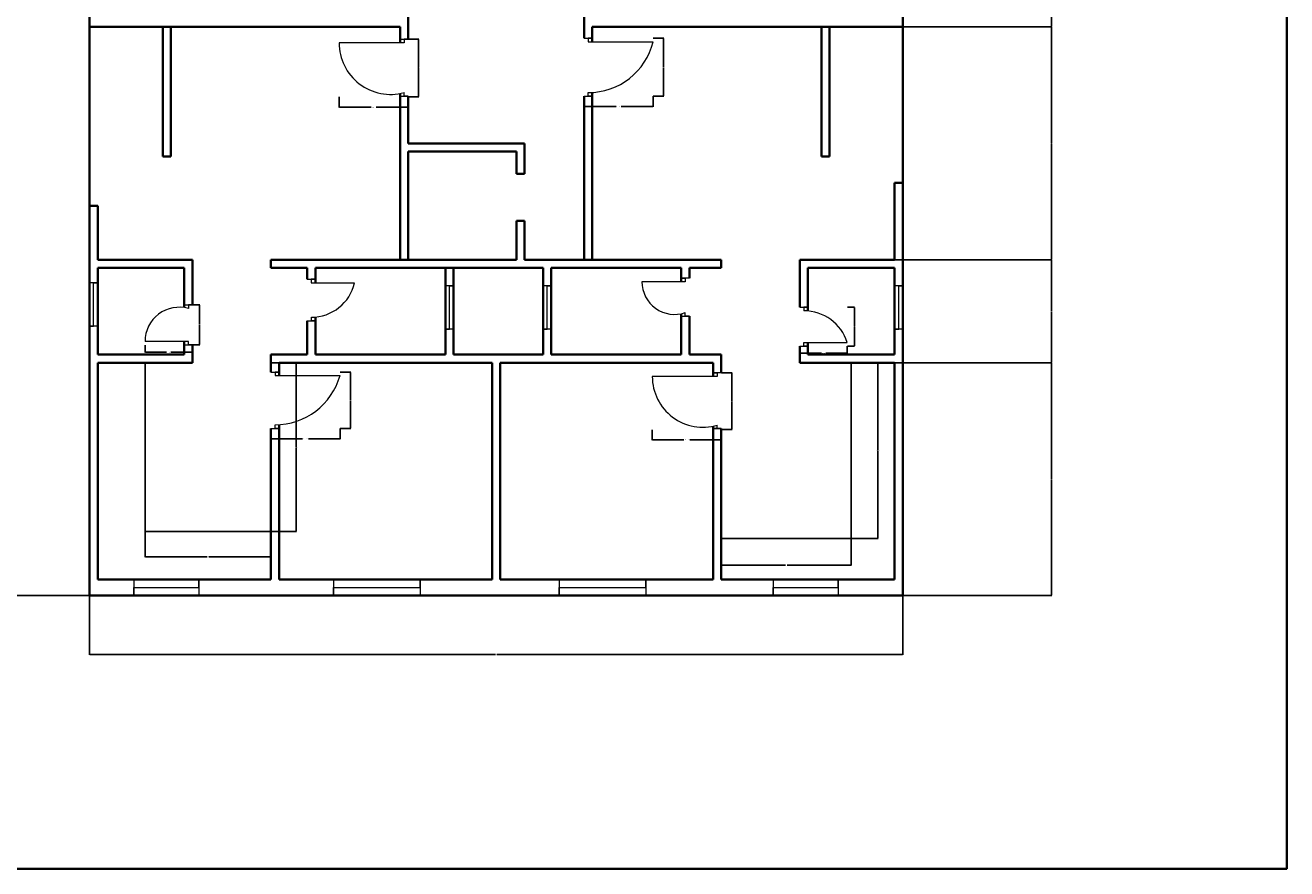
# Model space of a CAD drawing. Units: inches. Extents: x 2043 to 3387, y 1535 to 2797.
# Tile 4 of 7: x 2688 to 3387, y 1535 to 2002. Entities that reach past the tile are written whole.
import ezdxf

# ---------------------------------------------------------------- set-up
doc = ezdxf.new("R2010")
doc.units = ezdxf.units.IN
for name, color, linetype, lineweight in [('A-ANNO-DIMS', 2, 'Continuous', 18), ('A-ANNO-TTLB', 7, 'Continuous', 35), ('A-DOOR', 3, 'Continuous', 18), ('A-FLOR-FIXT', 9, 'Continuous', 25), ('A-GLAZ', 4, 'Continuous', 18), ('A-WALL', 7, 'Continuous', 35)]:
    doc.layers.add(name, color=color, linetype=linetype, lineweight=lineweight)
doc.styles.get("Standard").update_dxf_attribs({"font": 'arial.ttf'})
doc.dimstyles.get("Standard").update_dxf_attribs({"dimtxt": 0.18, "dimasz": 0.18, "dimexe": 0.18, "dimexo": 0.0625, "dimgap": 0.09, "dimtad": 0, "dimtih": 1, "dimtoh": 1, "dimdec": 4, "dimzin": 0, "dimdsep": 46, "dimtxsty": 'Standard', "dimcen": 0.09, "dimadec": 0, "dimazin": 0, "dimtfac": 1, "dimtdec": 4, "dimtofl": 0, "dimtmove": 0, "dimatfit": 3, "dimfxl": 1, "dimtolj": 1, "dimtzin": 0, "dimarcsym": 0})

# ---------------------------------------------------------------- blocks, each defined once
blk = doc.blocks.new('DOOR-36-ENTRY-SW')
for p, q in [((36, 29.57), (0, 29.57)), ((33.75, 31.57), (38.25, 31.57)), ((38.25, 31.57), (36, 31.57)), ((36, 31.57), (36, 29.57)), ((36, 0), (36, 2)), ((33.75, 0), (38.25, 0)), ((38.25, 0), (36, 0))]:
    blk.add_line(p, q)
blk.add_arc((28.56, 29.57), 28.56, 180, 285.10352)
blk = doc.blocks.new('DOOR-36-ENTRY-SE')
for p, q in [((0, 32.19), (4.5, 32.19)), ((4.5, 32.19), (2.25, 32.19)), ((2.25, 32.19), (2.25, 30.19)), ((2.25, 30.19), (38.25, 30.19)), ((2.25, 0), (2.25, 2)), ((0, 0), (4.5, 0)), ((4.5, 0), (2.25, 0))]:
    blk.add_line(p, q)
blk.add_arc((2.25, 39.08), 37.08, 270, 346.11724)
blk = doc.blocks.new('DOOR-24-WC-SW')
for p, q in [((21.75, 22.19), (26.25, 22.19)), ((26.25, 22.19), (24, 22.19)), ((24, 22.19), (24, 20.19)), ((24, 2), (0, 2)), ((21.75, 0), (26.25, 0)), ((24, 0), (24, 2)), ((26.25, 0), (24, 0))]:
    blk.add_line(p, q)
blk.add_arc((18.89, 2), 18.89, 74.30449, 180)
blk = doc.blocks.new('DOOR-24-BATH-SW')
for p, q in [((0, 23.05), (4.63, 23.05)), ((4.63, 23.05), (2.31, 23.05)), ((2.31, 23.05), (2.31, 21.05)), ((2.31, 21.05), (26.31, 21.05)), ((2.34, 0), (2.34, 2)), ((0.06, 0), (4.63, 0)), ((4.63, 0), (2.34, 0))]:
    blk.add_line(p, q)
blk.add_arc((2.34, 26.6), 24.6, 270, 346.95638)
blk = doc.blocks.new('DOOR-24-BATH-SE')
for p, q in [((26.25, 21.13), (21.75, 21.13)), ((21.75, 21.13), (24, 21.13)), ((24, 21.13), (24, 19.13)), ((24, 19.13), (0, 19.13)), ((24, 0), (24, 2)), ((21.75, 0), (26.25, 0)), ((26.25, 0), (24, 0))]:
    blk.add_line(p, q)
blk.add_arc((18.12, 19.13), 18.12, 180, 288.95077)
blk = doc.blocks.new('DOOR-24-WC-SE')
for p, q in [((0, 21.53), (4.5, 21.53)), ((4.5, 21.53), (2.25, 21.53)), ((2.25, 21.53), (2.25, 19.53)), ((0, 0), (4.5, 0)), ((2.25, 0), (2.25, 2)), ((2.25, 2), (26.25, 2)), ((4.5, 0), (2.25, 0))]:
    blk.add_line(p, q)
blk.add_arc((2.25, -5.66), 25.19, 17.71019, 90)
blk = doc.blocks.new('DOOR-36-BED-SE')
for p, q in [((36, 28.83), (0, 28.83)), ((38.25, 30.83), (33.75, 30.83)), ((33.75, 30.83), (36, 30.83)), ((36, 30.83), (36, 28.83)), ((33.75, 0), (38.25, 0)), ((38.25, 0), (33.75, 0)), ((33.75, 0), (36, 0)), ((36, 0), (36, 2))]:
    blk.add_line(p, q)
blk.add_arc((28, 28.83), 28, 180, 286.60822)
blk = doc.blocks.new('DOOR-36-BED-SW')
for p, q in [((0, 31.2), (4.5, 31.2)), ((4.5, 31.2), (2.25, 31.2)), ((2.25, 31.2), (2.25, 29.2)), ((2.25, 29.2), (38.25, 29.2)), ((0, 0), (4.5, 0)), ((2.25, 0), (2.25, 2)), ((4.5, 0), (2.25, 0))]:
    blk.add_line(p, q)
blk.add_arc((2.25, 39.42), 37.42, 270, 344.14237)
blk = doc.blocks.new('COUNTER-L-SW')
for p, q in [((0, 93.54), (0, 0)), ((0, 0), (69.75, 0))]:
    blk.add_line(p, q)
blk = doc.blocks.new('COUNTER-L-SE')
for p, q in [((72, 97.45), (72, 0)), ((72, 0), (0, 0))]:
    blk.add_line(p, q)
blk = doc.blocks.new('WIN-48-PLAN')
for p, q in [((0, 9), (0, 0)), ((48, 4.5), (48, 9)), ((48, 9), (48, 0)), ((0, 0), (0, 4.5)), ((0, 4.5), (48, 4.5))]:
    blk.add_line(p, q)
blk = doc.blocks.new('VENT-24-PLAN')
for p, q in [((0, 24), (4.5, 24)), ((4.5, 24), (2.25, 24)), ((2.25, 24), (2.25, 0)), ((2.25, 0), (0, 0)), ((0, 0), (4.5, 0))]:
    blk.add_line(p, q)
blk = doc.blocks.new('WIN-36-PLAN')
for p, q in [((0, 9), (0, 0)), ((36, 4.5), (36, 9)), ((36, 9), (36, 0)), ((0, 0), (0, 4.5)), ((0, 4.5), (36, 4.5))]:
    blk.add_line(p, q)
blk = doc.blocks.new('*D53')
at = {"layer": 'A-ANNO-DIMS', "color": 0, "lineweight": -2, "transparency": 16777216}
for p, q in [((2754.46, 1824.65), (2754.46, 1820.59)), ((2780.71, 1824.65), (2780.71, 1820.59)), ((2754.64, 1820.77), (2766.4, 1820.77)), ((2780.53, 1820.77), (2768.77, 1820.77))]:
    blk.add_line(p, q, dxfattribs=at)
at = {"layer": 'A-ANNO-DIMS', "color": 0, "transparency": 16777216}
for points in [[(2754.64, 1820.8), (2754.64, 1820.74), (2754.46, 1820.77)], [(2780.53, 1820.8), (2780.53, 1820.74), (2780.71, 1820.77)]]:
    blk.add_solid(points, dxfattribs=at)
at = {"layer": 'Defpoints', "color": 0, "transparency": 16777216}
for p in [(2754.46, 1824.71), (2780.71, 1824.71), (2780.71, 1820.77)]:
    blk.add_point(p, dxfattribs=at)
at = {"layer": 'A-ANNO-DIMS', "color": 0, "transparency": 16777216, "insert": (2767.58, 1820.77), "char_height": 0.18, "attachment_point": 5}
blk.add_mtext('\\A1;WC DOOR 26 TYP.', dxfattribs=at)
blk = doc.blocks.new('*D54')
at = {"layer": 'A-ANNO-DIMS', "color": 0, "lineweight": -2, "transparency": 16777216}
for p, q in [((2780.77, 1846.9), (2784.83, 1846.9)), ((2784.65, 1846.72), (2784.65, 1835.98)), ((2784.65, 1824.89), (2784.65, 1835.62)), ((2780.77, 1824.71), (2784.83, 1824.71))]:
    blk.add_line(p, q, dxfattribs=at)
at = {"layer": 'A-ANNO-DIMS', "color": 0, "transparency": 16777216}
for points in [[(2784.62, 1846.72), (2784.68, 1846.72), (2784.65, 1846.9)], [(2784.62, 1824.89), (2784.68, 1824.89), (2784.65, 1824.71)]]:
    blk.add_solid(points, dxfattribs=at)
at = {"layer": 'Defpoints', "color": 0, "transparency": 16777216}
for p in [(2780.71, 1846.9), (2784.65, 1846.9), (2780.71, 1824.71)]:
    blk.add_point(p, dxfattribs=at)
at = {"layer": 'A-ANNO-DIMS', "color": 0, "transparency": 16777216, "insert": (2784.65, 1835.8), "char_height": 0.18, "attachment_point": 5}
blk.add_mtext('\\A1;22 TYP.', dxfattribs=at)
blk = doc.blocks.new('*D55')
at = {"layer": 'A-ANNO-DIMS', "color": 0, "lineweight": -2, "transparency": 16777216}
for p, q in [((3117.21, 1824.03), (3117.21, 1819.98)), ((3117.39, 1820.16), (3129.15, 1820.16)), ((3143.28, 1820.16), (3131.52, 1820.16)), ((3143.46, 1824.03), (3143.46, 1819.98))]:
    blk.add_line(p, q, dxfattribs=at)
at = {"layer": 'A-ANNO-DIMS', "color": 0, "transparency": 16777216}
for points in [[(3117.39, 1820.19), (3117.39, 1820.13), (3117.21, 1820.16)], [(3143.28, 1820.19), (3143.28, 1820.13), (3143.46, 1820.16)]]:
    blk.add_solid(points, dxfattribs=at)
at = {"layer": 'Defpoints', "color": 0, "transparency": 16777216}
for p in [(3117.21, 1824.1), (3143.46, 1824.1), (3143.46, 1820.16)]:
    blk.add_point(p, dxfattribs=at)
at = {"layer": 'A-ANNO-DIMS', "color": 0, "transparency": 16777216, "insert": (3130.33, 1820.16), "char_height": 0.18, "attachment_point": 5}
blk.add_mtext('\\A1;WC DOOR 26 TYP.', dxfattribs=at)
blk = doc.blocks.new('*D56')
at = {"layer": 'A-ANNO-DIMS', "color": 0, "lineweight": -2, "transparency": 16777216}
for p, q in [((3143.52, 1845.63), (3147.58, 1845.63)), ((3147.4, 1845.45), (3147.4, 1835.04)), ((3147.4, 1824.28), (3147.4, 1834.68)), ((3143.52, 1824.1), (3147.58, 1824.1))]:
    blk.add_line(p, q, dxfattribs=at)
at = {"layer": 'A-ANNO-DIMS', "color": 0, "transparency": 16777216}
for points in [[(3147.37, 1845.45), (3147.43, 1845.45), (3147.4, 1845.63)], [(3147.37, 1824.28), (3147.43, 1824.28), (3147.4, 1824.1)]]:
    blk.add_solid(points, dxfattribs=at)
at = {"layer": 'Defpoints', "color": 0, "transparency": 16777216}
for p in [(3143.46, 1845.63), (3147.4, 1845.63), (3143.46, 1824.1)]:
    blk.add_point(p, dxfattribs=at)
at = {"layer": 'A-ANNO-DIMS', "color": 0, "transparency": 16777216, "insert": (3147.4, 1834.86), "char_height": 0.18, "attachment_point": 5}
blk.add_mtext('\\A1;22 TYP.', dxfattribs=at)
blk = doc.blocks.new('*D69')
at = {"layer": 'A-ANNO-DIMS', "color": 0, "lineweight": -2, "transparency": 16777216}
for p, q in [((2861.96, 1962.12), (2861.96, 1956.27)), ((2900.21, 1962.12), (2900.21, 1956.27)), ((2862.14, 1956.45), (2879.69, 1956.45)), ((2900.03, 1956.45), (2882.48, 1956.45))]:
    blk.add_line(p, q, dxfattribs=at)
at = {"layer": 'A-ANNO-DIMS', "color": 0, "transparency": 16777216}
for points in [[(2862.14, 1956.48), (2862.14, 1956.42), (2861.96, 1956.45)], [(2900.03, 1956.48), (2900.03, 1956.42), (2900.21, 1956.45)]]:
    blk.add_solid(points, dxfattribs=at)
at = {"layer": 'Defpoints', "color": 0, "transparency": 16777216}
for p in [(2861.96, 1962.19), (2900.21, 1962.19), (2900.21, 1956.45)]:
    blk.add_point(p, dxfattribs=at)
at = {"layer": 'A-ANNO-DIMS', "color": 0, "transparency": 16777216, "insert": (2881.08, 1956.45), "char_height": 0.18, "attachment_point": 5}
blk.add_mtext('\\A1;ENTRY DOOR 38 TYP.', dxfattribs=at)
blk = doc.blocks.new('*D70')
at = {"layer": 'A-ANNO-DIMS', "color": 0, "lineweight": -2, "transparency": 16777216}
for p, q in [((2900.27, 1994.07), (2906.13, 1994.07)), ((2905.95, 1993.89), (2905.95, 1978.31)), ((2905.95, 1962.37), (2905.95, 1977.95)), ((2900.27, 1962.19), (2906.13, 1962.19))]:
    blk.add_line(p, q, dxfattribs=at)
at = {"layer": 'A-ANNO-DIMS', "color": 0, "transparency": 16777216}
for points in [[(2905.92, 1993.89), (2905.98, 1993.89), (2905.95, 1994.07)], [(2905.92, 1962.37), (2905.98, 1962.37), (2905.95, 1962.19)]]:
    blk.add_solid(points, dxfattribs=at)
at = {"layer": 'Defpoints', "color": 0, "transparency": 16777216}
for p in [(2900.21, 1994.07), (2905.95, 1994.07), (2900.21, 1962.19)]:
    blk.add_point(p, dxfattribs=at)
at = {"layer": 'A-ANNO-DIMS', "color": 0, "transparency": 16777216, "insert": (2905.95, 1978.13), "char_height": 0.18, "attachment_point": 5}
blk.add_mtext('\\A1;32 TYP.', dxfattribs=at)
blk = doc.blocks.new('*D71')
at = {"layer": 'A-ANNO-DIMS', "color": 0, "lineweight": -2, "transparency": 16777216}
for p, q in [((2997.71, 1962.44), (2997.71, 1956.58)), ((3035.96, 1962.44), (3035.96, 1956.58)), ((2997.89, 1956.76), (3015.44, 1956.76)), ((3035.78, 1956.76), (3018.23, 1956.76))]:
    blk.add_line(p, q, dxfattribs=at)
at = {"layer": 'A-ANNO-DIMS', "color": 0, "transparency": 16777216}
for points in [[(2997.89, 1956.79), (2997.89, 1956.73), (2997.71, 1956.76)], [(3035.78, 1956.79), (3035.78, 1956.73), (3035.96, 1956.76)]]:
    blk.add_solid(points, dxfattribs=at)
at = {"layer": 'Defpoints', "color": 0, "transparency": 16777216}
for p in [(2997.71, 1962.5), (3035.96, 1962.5), (3035.96, 1956.76)]:
    blk.add_point(p, dxfattribs=at)
at = {"layer": 'A-ANNO-DIMS', "color": 0, "transparency": 16777216, "insert": (3016.83, 1956.76), "char_height": 0.18, "attachment_point": 5}
blk.add_mtext('\\A1;ENTRY DOOR 38 TYP.', dxfattribs=at)
blk = doc.blocks.new('*D72')
at = {"layer": 'A-ANNO-DIMS', "color": 0, "lineweight": -2, "transparency": 16777216}
for p, q in [((3036.02, 1994.69), (3041.88, 1994.69)), ((3041.7, 1994.51), (3041.7, 1978.78)), ((3041.7, 1962.68), (3041.7, 1978.41)), ((3036.02, 1962.5), (3041.88, 1962.5))]:
    blk.add_line(p, q, dxfattribs=at)
at = {"layer": 'A-ANNO-DIMS', "color": 0, "transparency": 16777216}
for points in [[(3041.67, 1994.51), (3041.73, 1994.51), (3041.7, 1994.69)], [(3041.67, 1962.68), (3041.73, 1962.68), (3041.7, 1962.5)]]:
    blk.add_solid(points, dxfattribs=at)
at = {"layer": 'Defpoints', "color": 0, "transparency": 16777216}
for p in [(3035.96, 1994.69), (3041.7, 1994.69), (3035.96, 1962.5)]:
    blk.add_point(p, dxfattribs=at)
at = {"layer": 'A-ANNO-DIMS', "color": 0, "transparency": 16777216, "insert": (3041.7, 1978.59), "char_height": 0.18, "attachment_point": 5}
blk.add_mtext('\\A1;32 TYP.', dxfattribs=at)
blk = doc.blocks.new('*D77')
at = {"layer": 'A-ANNO-DIMS', "color": 0, "lineweight": -2, "transparency": 16777216}
for p, q in [((2824.21, 1778.46), (2824.21, 1772.61)), ((2862.46, 1778.46), (2862.46, 1772.61)), ((2824.39, 1772.79), (2841.71, 1772.79)), ((2862.28, 1772.79), (2844.95, 1772.79))]:
    blk.add_line(p, q, dxfattribs=at)
at = {"layer": 'A-ANNO-DIMS', "color": 0, "transparency": 16777216}
for points in [[(2824.39, 1772.82), (2824.39, 1772.76), (2824.21, 1772.79)], [(2862.28, 1772.82), (2862.28, 1772.76), (2862.46, 1772.79)]]:
    blk.add_solid(points, dxfattribs=at)
at = {"layer": 'Defpoints', "color": 0, "transparency": 16777216}
for p in [(2824.21, 1778.52), (2862.46, 1778.52), (2862.46, 1772.79)]:
    blk.add_point(p, dxfattribs=at)
at = {"layer": 'A-ANNO-DIMS', "color": 0, "transparency": 16777216, "insert": (2843.33, 1772.79), "char_height": 0.18, "attachment_point": 5}
blk.add_mtext('\\A1;BEDROOM DOOR 38 TYP.', dxfattribs=at)
blk = doc.blocks.new('*D78')
at = {"layer": 'A-ANNO-DIMS', "color": 0, "lineweight": -2, "transparency": 16777216}
for p, q in [((2862.52, 1809.72), (2868.38, 1809.72)), ((2868.2, 1809.54), (2868.2, 1794.3)), ((2868.2, 1778.7), (2868.2, 1793.94)), ((2862.52, 1778.52), (2868.38, 1778.52))]:
    blk.add_line(p, q, dxfattribs=at)
at = {"layer": 'A-ANNO-DIMS', "color": 0, "transparency": 16777216}
for points in [[(2868.17, 1809.54), (2868.23, 1809.54), (2868.2, 1809.72)], [(2868.17, 1778.7), (2868.23, 1778.7), (2868.2, 1778.52)]]:
    blk.add_solid(points, dxfattribs=at)
at = {"layer": 'Defpoints', "color": 0, "transparency": 16777216}
for p in [(2862.46, 1809.72), (2868.2, 1809.72), (2862.46, 1778.52)]:
    blk.add_point(p, dxfattribs=at)
at = {"layer": 'A-ANNO-DIMS', "color": 0, "transparency": 16777216, "insert": (2868.2, 1794.12), "char_height": 0.18, "attachment_point": 5}
blk.add_mtext('\\A1;31 TYP.', dxfattribs=at)
blk = doc.blocks.new('*D79')
at = {"layer": 'A-ANNO-DIMS', "color": 0, "lineweight": -2, "transparency": 16777216}
for p, q in [((3035.46, 1777.76), (3035.46, 1771.91)), ((3073.71, 1777.76), (3073.71, 1771.91)), ((3035.64, 1772.09), (3052.96, 1772.09)), ((3073.53, 1772.09), (3056.2, 1772.09))]:
    blk.add_line(p, q, dxfattribs=at)
at = {"layer": 'A-ANNO-DIMS', "color": 0, "transparency": 16777216}
for points in [[(3035.64, 1772.12), (3035.64, 1772.06), (3035.46, 1772.09)], [(3073.53, 1772.12), (3073.53, 1772.06), (3073.71, 1772.09)]]:
    blk.add_solid(points, dxfattribs=at)
at = {"layer": 'Defpoints', "color": 0, "transparency": 16777216}
for p in [(3035.46, 1777.82), (3073.71, 1777.82), (3073.71, 1772.09)]:
    blk.add_point(p, dxfattribs=at)
at = {"layer": 'A-ANNO-DIMS', "color": 0, "transparency": 16777216, "insert": (3054.58, 1772.09), "char_height": 0.18, "attachment_point": 5}
blk.add_mtext('\\A1;BEDROOM DOOR 38 TYP.', dxfattribs=at)
blk = doc.blocks.new('*D80')
at = {"layer": 'A-ANNO-DIMS', "color": 0, "lineweight": -2, "transparency": 16777216}
for p, q in [((3073.77, 1809.18), (3079.63, 1809.18)), ((3079.45, 1809), (3079.45, 1793.69)), ((3079.45, 1778), (3079.45, 1793.32)), ((3073.77, 1777.82), (3079.63, 1777.82))]:
    blk.add_line(p, q, dxfattribs=at)
at = {"layer": 'A-ANNO-DIMS', "color": 0, "transparency": 16777216}
for points in [[(3079.42, 1809), (3079.48, 1809), (3079.45, 1809.18)], [(3079.42, 1778), (3079.48, 1778), (3079.45, 1777.82)]]:
    blk.add_solid(points, dxfattribs=at)
at = {"layer": 'Defpoints', "color": 0, "transparency": 16777216}
for p in [(3073.71, 1809.18), (3079.45, 1809.18), (3073.71, 1777.82)]:
    blk.add_point(p, dxfattribs=at)
at = {"layer": 'A-ANNO-DIMS', "color": 0, "transparency": 16777216, "insert": (3079.45, 1793.5), "char_height": 0.18, "attachment_point": 5}
blk.add_mtext('\\A1;31 TYP.', dxfattribs=at)
blk = doc.blocks.new('*D85')
at = {"layer": 'A-ANNO-DIMS', "color": 0, "lineweight": -2, "transparency": 16777216}
for p, q in [((2824.27, 1814.88), (2838.42, 1814.88)), ((2838.24, 1814.7), (2838.24, 1768.29)), ((2838.24, 1721.52), (2838.24, 1767.92)), ((2824.27, 1721.34), (2838.42, 1721.34))]:
    blk.add_line(p, q, dxfattribs=at)
at = {"layer": 'A-ANNO-DIMS', "color": 0, "transparency": 16777216}
for points in [[(2838.21, 1814.7), (2838.27, 1814.7), (2838.24, 1814.88)], [(2838.21, 1721.52), (2838.27, 1721.52), (2838.24, 1721.34)]]:
    blk.add_solid(points, dxfattribs=at)
at = {"layer": 'Defpoints', "color": 0, "transparency": 16777216}
for p in [(2824.21, 1814.88), (2838.24, 1814.88), (2824.21, 1721.34)]:
    blk.add_point(p, dxfattribs=at)
at = {"layer": 'A-ANNO-DIMS', "color": 0, "transparency": 16777216, "insert": (2838.24, 1768.11), "char_height": 0.18, "attachment_point": 5}
blk.add_mtext('\\A1;COUNTER 94 TYP.', dxfattribs=at)
blk = doc.blocks.new('*D86')
at = {"layer": 'A-ANNO-DIMS', "color": 0, "lineweight": -2, "transparency": 16777216}
for p, q in [((2754.46, 1721.28), (2754.46, 1707.13)), ((2824.21, 1721.28), (2824.21, 1707.13)), ((2754.64, 1707.31), (2788.81, 1707.31)), ((2824.03, 1707.31), (2789.86, 1707.31))]:
    blk.add_line(p, q, dxfattribs=at)
at = {"layer": 'A-ANNO-DIMS', "color": 0, "transparency": 16777216}
for points in [[(2754.64, 1707.34), (2754.64, 1707.28), (2754.46, 1707.31)], [(2824.03, 1707.34), (2824.03, 1707.28), (2824.21, 1707.31)]]:
    blk.add_solid(points, dxfattribs=at)
at = {"layer": 'Defpoints', "color": 0, "transparency": 16777216}
for p in [(2754.46, 1721.34), (2824.21, 1721.34), (2824.21, 1707.31)]:
    blk.add_point(p, dxfattribs=at)
at = {"layer": 'A-ANNO-DIMS', "color": 0, "transparency": 16777216, "insert": (2789.33, 1707.31), "char_height": 0.18, "attachment_point": 5}
blk.add_mtext('\\A1;70 TYP.', dxfattribs=at)
blk = doc.blocks.new('*D87')
at = {"layer": 'A-ANNO-DIMS', "color": 0, "lineweight": -2, "transparency": 16777216}
for p, q in [((3145.77, 1814.88), (3160.51, 1814.88)), ((3160.33, 1814.7), (3160.33, 1766.33)), ((3160.33, 1717.6), (3160.33, 1765.97)), ((3145.77, 1717.42), (3160.51, 1717.42))]:
    blk.add_line(p, q, dxfattribs=at)
at = {"layer": 'A-ANNO-DIMS', "color": 0, "transparency": 16777216}
for points in [[(3160.3, 1814.7), (3160.36, 1814.7), (3160.33, 1814.88)], [(3160.3, 1717.6), (3160.36, 1717.6), (3160.33, 1717.42)]]:
    blk.add_solid(points, dxfattribs=at)
at = {"layer": 'Defpoints', "color": 0, "transparency": 16777216}
for p in [(3145.71, 1814.88), (3160.33, 1814.88), (3145.71, 1717.42)]:
    blk.add_point(p, dxfattribs=at)
at = {"layer": 'A-ANNO-DIMS', "color": 0, "transparency": 16777216, "insert": (3160.33, 1766.15), "char_height": 0.18, "attachment_point": 5}
blk.add_mtext('\\A1;COUNTER 97 TYP.', dxfattribs=at)
blk = doc.blocks.new('*D88')
at = {"layer": 'A-ANNO-DIMS', "color": 0, "lineweight": -2, "transparency": 16777216}
for p, q in [((3073.71, 1717.36), (3073.71, 1702.62)), ((3145.71, 1717.36), (3145.71, 1702.62)), ((3073.89, 1702.8), (3109.18, 1702.8)), ((3145.53, 1702.8), (3110.24, 1702.8))]:
    blk.add_line(p, q, dxfattribs=at)
at = {"layer": 'A-ANNO-DIMS', "color": 0, "transparency": 16777216}
for points in [[(3073.89, 1702.83), (3073.89, 1702.77), (3073.71, 1702.8)], [(3145.53, 1702.83), (3145.53, 1702.77), (3145.71, 1702.8)]]:
    blk.add_solid(points, dxfattribs=at)
at = {"layer": 'Defpoints', "color": 0, "transparency": 16777216}
for p in [(3073.71, 1717.42), (3145.71, 1717.42), (3145.71, 1702.8)]:
    blk.add_point(p, dxfattribs=at)
at = {"layer": 'A-ANNO-DIMS', "color": 0, "transparency": 16777216, "insert": (3109.71, 1702.8), "char_height": 0.18, "attachment_point": 5}
blk.add_mtext('\\A1;72 TYP.', dxfattribs=at)
blk = doc.blocks.new('*D105')
at = {"layer": 'A-ANNO-DIMS', "color": 0, "lineweight": -2, "transparency": 16777216}
for p, q in [((2723.71, 1685.81), (2723.71, 1653)), ((3174.21, 1685.81), (3174.21, 1653)), ((2723.89, 1653.18), (2948.56, 1653.18)), ((3174.03, 1653.18), (2949.36, 1653.18))]:
    blk.add_line(p, q, dxfattribs=at)
at = {"layer": 'A-ANNO-DIMS', "color": 0, "transparency": 16777216}
for points in [[(2723.89, 1653.21), (2723.89, 1653.15), (2723.71, 1653.18)], [(3174.03, 1653.21), (3174.03, 1653.15), (3174.21, 1653.18)]]:
    blk.add_solid(points, dxfattribs=at)
at = {"layer": 'Defpoints', "color": 0, "transparency": 16777216}
for p in [(2723.71, 1685.88), (3174.21, 1685.88), (3174.21, 1653.18)]:
    blk.add_point(p, dxfattribs=at)
at = {"layer": 'A-ANNO-DIMS', "color": 0, "transparency": 16777216, "insert": (2948.96, 1653.18), "char_height": 0.18, "attachment_point": 5}
blk.add_mtext('\\A1;450.5', dxfattribs=at)
blk = doc.blocks.new('*D106')
at = {"layer": 'A-ANNO-DIMS', "color": 0, "lineweight": -2, "transparency": 16777216}
for p, q in [((2723.65, 2326.38), (2660.13, 2326.38)), ((2660.31, 2326.2), (2660.31, 2006.31)), ((2660.31, 1686.06), (2660.31, 2005.95)), ((2723.65, 1685.88), (2660.13, 1685.88))]:
    blk.add_line(p, q, dxfattribs=at)
at = {"layer": 'A-ANNO-DIMS', "color": 0, "transparency": 16777216}
for points in [[(2660.28, 2326.2), (2660.34, 2326.2), (2660.31, 2326.38)], [(2660.28, 1686.06), (2660.34, 1686.06), (2660.31, 1685.88)]]:
    blk.add_solid(points, dxfattribs=at)
at = {"layer": 'Defpoints', "color": 0, "transparency": 16777216}
for p in [(2660.31, 2326.38), (2723.71, 2326.38), (2723.71, 1685.88)]:
    blk.add_point(p, dxfattribs=at)
at = {"layer": 'A-ANNO-DIMS', "color": 0, "transparency": 16777216, "insert": (2660.31, 2006.13), "char_height": 0.18, "attachment_point": 5}
blk.add_mtext('\\A1;640.5', dxfattribs=at)
blk = doc.blocks.new('*D111')
at = {"layer": 'A-ANNO-DIMS', "color": 0, "lineweight": -2, "transparency": 16777216}
for p, q in [((3169.77, 1814.88), (3256.85, 1814.88)), ((3256.67, 1814.7), (3256.67, 1750.56)), ((3256.67, 1686.06), (3256.67, 1750.2)), ((3174.27, 1685.88), (3256.85, 1685.88))]:
    blk.add_line(p, q, dxfattribs=at)
at = {"layer": 'A-ANNO-DIMS', "color": 0, "transparency": 16777216}
for points in [[(3256.64, 1814.7), (3256.7, 1814.7), (3256.67, 1814.88)], [(3256.64, 1686.06), (3256.7, 1686.06), (3256.67, 1685.88)]]:
    blk.add_solid(points, dxfattribs=at)
at = {"layer": 'Defpoints', "color": 0, "transparency": 16777216}
for p in [(3169.71, 1814.88), (3256.67, 1814.88), (3174.21, 1685.88)]:
    blk.add_point(p, dxfattribs=at)
at = {"layer": 'A-ANNO-DIMS', "color": 0, "transparency": 16777216, "insert": (3256.67, 1750.38), "char_height": 0.18, "attachment_point": 5}
blk.add_mtext('\\A1;129', dxfattribs=at)
blk = doc.blocks.new('*D112')
at = {"layer": 'A-ANNO-DIMS', "color": 0, "lineweight": -2, "transparency": 16777216}
for p, q in [((3169.77, 1871.88), (3256.85, 1871.88)), ((3256.67, 1871.7), (3256.67, 1843.56)), ((3256.67, 1815.06), (3256.67, 1843.2)), ((3169.77, 1814.88), (3256.85, 1814.88))]:
    blk.add_line(p, q, dxfattribs=at)
at = {"layer": 'A-ANNO-DIMS', "color": 0, "transparency": 16777216}
for points in [[(3256.64, 1871.7), (3256.7, 1871.7), (3256.67, 1871.88)], [(3256.64, 1815.06), (3256.7, 1815.06), (3256.67, 1814.88)]]:
    blk.add_solid(points, dxfattribs=at)
at = {"layer": 'Defpoints', "color": 0, "transparency": 16777216}
for p in [(3169.71, 1871.88), (3256.67, 1871.88), (3169.71, 1814.88)]:
    blk.add_point(p, dxfattribs=at)
at = {"layer": 'A-ANNO-DIMS', "color": 0, "transparency": 16777216, "insert": (3256.67, 1843.38), "char_height": 0.18, "attachment_point": 5}
blk.add_mtext('\\A1;57', dxfattribs=at)
blk = doc.blocks.new('*D113')
at = {"layer": 'A-ANNO-DIMS', "color": 0, "lineweight": -2, "transparency": 16777216}
for p, q in [((3174.27, 2000.88), (3256.85, 2000.88)), ((3256.67, 2000.7), (3256.67, 1936.56)), ((3256.67, 1872.06), (3256.67, 1936.2)), ((3169.77, 1871.88), (3256.85, 1871.88))]:
    blk.add_line(p, q, dxfattribs=at)
at = {"layer": 'A-ANNO-DIMS', "color": 0, "transparency": 16777216}
for points in [[(3256.64, 2000.7), (3256.7, 2000.7), (3256.67, 2000.88)], [(3256.64, 1872.06), (3256.7, 1872.06), (3256.67, 1871.88)]]:
    blk.add_solid(points, dxfattribs=at)
at = {"layer": 'Defpoints', "color": 0, "transparency": 16777216}
for p in [(3174.21, 2000.88), (3256.67, 2000.88), (3169.71, 1871.88)]:
    blk.add_point(p, dxfattribs=at)
at = {"layer": 'A-ANNO-DIMS', "color": 0, "transparency": 16777216, "insert": (3256.67, 1936.38), "char_height": 0.18, "attachment_point": 5}
blk.add_mtext('\\A1;129', dxfattribs=at)
blk = doc.blocks.new('*D114')
at = {"layer": 'A-ANNO-DIMS', "color": 0, "lineweight": -2, "transparency": 16777216}
for p, q in [((3169.77, 2134.38), (3256.85, 2134.38)), ((3256.67, 2134.2), (3256.67, 2067.81)), ((3256.67, 2001.06), (3256.67, 2067.44)), ((3174.27, 2000.88), (3256.85, 2000.88))]:
    blk.add_line(p, q, dxfattribs=at)
at = {"layer": 'A-ANNO-DIMS', "color": 0, "transparency": 16777216}
for points in [[(3256.64, 2134.2), (3256.7, 2134.2), (3256.67, 2134.38)], [(3256.64, 2001.06), (3256.7, 2001.06), (3256.67, 2000.88)]]:
    blk.add_solid(points, dxfattribs=at)
at = {"layer": 'Defpoints', "color": 0, "transparency": 16777216}
for p in [(3169.71, 2134.38), (3256.67, 2134.38), (3174.21, 2000.88)]:
    blk.add_point(p, dxfattribs=at)
at = {"layer": 'A-ANNO-DIMS', "color": 0, "transparency": 16777216, "insert": (3256.67, 2067.63), "char_height": 0.18, "attachment_point": 5}
blk.add_mtext('\\A1;133.5', dxfattribs=at)

msp = doc.modelspace()

# ---------------------------------------------------------------- linework, layer by layer
at = {"layer": 'A-ANNO-TTLB'}
msp.add_lwpolyline([(2042.5541, 2796.7818), (3386.9704, 2796.7818), (3386.9704, 1534.5689), (2042.5541, 1534.5689)], close=True, dxfattribs=at)
at = {"layer": 'A-WALL'}
for p, q in [((2723.7086, 2326.3769), (2723.7086, 1734.4589)), ((3174.2086, 2326.3769), (3174.2086, 1685.8769)), ((2900.2086, 2009.0461), (2900.2086, 1994.0737)), ((2997.7086, 1994.6872), (2997.7086, 2009.4195)), ((2728.2086, 2000.8769), (2723.7086, 2000.8769)), ((2728.2086, 2000.8769), (2895.7086, 2000.8769)), ((2764.2086, 2000.8769), (2764.2086, 1929.0247)), ((2768.7086, 2000.8769), (2768.7086, 1929.0247)), ((2895.7086, 2000.8769), (2895.7086, 1992.0737)), ((3002.2086, 2000.8769), (3174.2086, 2000.8769)), ((3002.2086, 1992.6872), (3002.2086, 2000.8769)), ((3129.2086, 1929.0247), (3129.2086, 2000.8769)), ((3133.7086, 2000.8769), (3133.7086, 1929.0247)), ((2895.7086, 1963.9908), (2895.7086, 1871.8769)), ((3002.2086, 1871.8769), (3002.2086, 1964.5698)), ((2900.2086, 1962.5015), (2900.2086, 1936.3769)), ((2997.7086, 1871.8769), (2997.7086, 1962.5015)), ((2964.7086, 1936.3769), (2900.2086, 1936.3769)), ((2964.7086, 1931.8769), (2964.7086, 1936.3769)), ((2764.2086, 1929.0247), (2768.7086, 1929.0247)), ((2900.2086, 1931.8769), (2900.2086, 1871.8769)), ((2900.2086, 1871.8769), (2900.2086, 1931.8769)), ((2900.2086, 1931.8769), (2960.2086, 1931.8769)), ((2960.2086, 1931.8769), (2960.2086, 1919.4326)), ((2964.7086, 1919.4326), (2964.7086, 1931.8769)), ((3129.2086, 1929.0247), (3133.7086, 1929.0247)), ((2964.7086, 1919.4326), (2960.2086, 1919.4326)), ((3169.7086, 1914.5613), (3169.7086, 1871.8769)), ((3169.7086, 1914.5613), (3174.2086, 1914.5613)), ((2728.2086, 1901.8538), (2723.7086, 1901.8538)), ((2728.2086, 1901.8538), (2728.2086, 1871.8769)), ((2960.2086, 1893.5445), (2960.2086, 1871.8769)), ((2964.7086, 1893.5445), (2960.2086, 1893.5445)), ((2964.7086, 1871.8769), (2964.7086, 1893.5445)), ((2728.2086, 1871.8769), (2780.7086, 1871.8769)), ((2728.2086, 1867.3769), (2776.2086, 1867.3769)), ((2728.2086, 1867.3769), (2728.2086, 1819.3769)), ((2776.2086, 1845.3823), (2776.2086, 1867.3769)), ((2780.7086, 1867.3769), (2780.7086, 1871.8769)), ((2780.7086, 1867.3769), (2780.7086, 1846.8958)), ((2824.2086, 1867.3769), (2824.2086, 1871.8769)), ((2824.2086, 1871.8769), (2824.5414, 1871.8769)), ((2824.5414, 1867.3769), (2824.2086, 1867.3769)), ((2824.5414, 1871.8769), (2960.2086, 1871.8769)), ((2824.5414, 1867.3769), (2844.2209, 1867.3769)), ((2844.2379, 1861.1284), (2844.2209, 1867.3769)), ((2848.8641, 1867.3769), (2974.9865, 1867.3769)), ((2848.8641, 1867.3769), (2848.8641, 1859.1284)), ((2920.8641, 1867.3769), (2920.8641, 1819.3769)), ((2925.3641, 1867.3769), (2925.3641, 1819.3769)), ((2964.7086, 1871.8769), (3073.7086, 1871.8769)), ((2974.9865, 1867.3769), (2974.9865, 1819.3769)), ((2979.4865, 1867.3769), (3051.4865, 1867.3769)), ((2979.4865, 1819.3769), (2979.4865, 1867.3769)), ((3051.4865, 1859.7561), (3051.4865, 1867.3769)), ((3055.9865, 1867.3769), (3073.7086, 1867.3769)), ((3055.9865, 1867.3769), (3055.9865, 1861.7561)), ((3073.7086, 1871.8769), (3073.7086, 1867.3769)), ((3117.2086, 1871.8769), (3169.7086, 1871.8769)), ((3117.2086, 1845.6269), (3117.2086, 1871.8769)), ((3121.7086, 1867.3769), (3169.7086, 1867.3769)), ((3169.7086, 1867.3769), (3121.7086, 1867.3769)), ((3121.7086, 1867.3769), (3121.7086, 1843.5263)), ((3169.7086, 1867.3769), (3169.7086, 1819.3769)), ((2848.8641, 1840.1838), (2848.8641, 1819.3769)), ((3051.4865, 1819.3769), (3051.4865, 1842.0077)), ((3055.9865, 1840.6215), (3055.9865, 1819.3769)), ((2844.3518, 1819.3769), (2844.3008, 1838.0778)), ((2776.2086, 1819.3769), (2776.2086, 1826.7103)), ((2780.7086, 1824.7103), (2780.7086, 1814.8769)), ((3121.7086, 1826.097), (3121.7086, 1819.3769)), ((2728.2086, 1819.3769), (2776.2086, 1819.3769)), ((2728.2086, 1819.3769), (2776.2086, 1819.3769)), ((2824.2086, 1814.8769), (2824.2086, 1819.3769)), ((2824.2086, 1819.3769), (2824.5414, 1819.3769)), ((2824.5414, 1819.3769), (2844.3518, 1819.3769)), ((2848.8641, 1819.3769), (2920.8641, 1819.3769)), ((2925.3641, 1819.3769), (2974.9865, 1819.3769)), ((2979.4865, 1819.3769), (3051.4865, 1819.3769)), ((3055.9865, 1819.3769), (3073.7086, 1819.3769)), ((3073.7086, 1819.3769), (3073.7086, 1814.8769)), ((3117.2086, 1819.3769), (3117.2086, 1824.097)), ((3117.2086, 1819.3769), (3117.2086, 1814.8769)), ((3121.7086, 1819.3769), (3169.7086, 1819.3769)), ((2728.2086, 1814.8769), (2780.7086, 1814.8769)), ((2728.2086, 1814.8769), (2728.2086, 1694.8769)), ((2824.2086, 1814.8769), (2824.2086, 1809.7212)), ((2828.7086, 1814.8769), (2946.7086, 1814.8769)), ((2828.7086, 1814.8769), (2828.7086, 1807.7212)), ((2848.8641, 1814.8769), (2844.3641, 1814.8769)), ((2946.7086, 1814.8769), (2946.7086, 1694.8769)), ((2951.2086, 1814.8769), (3069.2086, 1814.8769)), ((2951.2086, 1814.8769), (2951.2086, 1694.8769)), ((3055.9865, 1814.8769), (3051.4865, 1814.8769)), ((3069.2086, 1814.8769), (3069.2086, 1807.1819)), ((3073.7086, 1814.8769), (3073.7086, 1809.1819)), ((3117.2086, 1814.8769), (3169.7086, 1814.8769)), ((3169.7086, 1814.8769), (3169.7086, 1694.8769)), ((2824.2086, 1778.5231), (2824.2086, 1694.8769)), ((2828.7086, 1780.5908), (2828.7086, 1694.8769)), ((3069.2086, 1779.7816), (3069.2086, 1694.8769)), ((3073.7086, 1778.3523), (3073.7086, 1694.8769)), ((2723.7086, 1734.4589), (2723.7086, 1685.8769)), ((2728.2086, 1694.8769), (2824.2086, 1694.8769)), ((2828.7086, 1694.8769), (2946.7086, 1694.8769)), ((2951.2086, 1694.8769), (3069.2086, 1694.8769)), ((3073.7086, 1694.8769), (3169.7086, 1694.8769)), ((2723.7086, 1685.8769), (3174.2086, 1685.8769))]:
    msp.add_line(p, q, dxfattribs=at)

# ---------------------------------------------------------------- block references
at = {"layer": 'A-DOOR'}
for name, p in [('DOOR-36-ENTRY-SW', (2861.959, 1962.502)), ('DOOR-36-ENTRY-SE', (2997.709, 1962.502)), ('DOOR-24-BATH-SW', (2844.238, 1838.078)), ('DOOR-24-BATH-SE', (3029.737, 1840.622)), ('DOOR-24-WC-SW', (2754.459, 1824.71)), ('DOOR-24-WC-SE', (3117.209, 1824.097)), ('DOOR-36-BED-SW', (2824.209, 1778.523)), ('DOOR-36-BED-SE', (3035.459, 1778.352))]:
    msp.add_blockref(name, p, dxfattribs=at)
at = {"layer": 'A-FLOR-FIXT'}
for name, p in [('COUNTER-L-SW', (2754.459, 1721.339)), ('COUNTER-L-SE', (3073.709, 1717.422))]:
    msp.add_blockref(name, p, dxfattribs=at)
at = {"layer": 'A-GLAZ', "rotation": 180}
for p in [(2728.2082, 1859.1776), (2925.3637, 1857.5339), (2979.4861, 1857.5339), (3174.2082, 1857.3829)]:
    msp.add_blockref('VENT-24-PLAN', p, dxfattribs=at)
at = {"layer": 'A-GLAZ'}
for name, p in [('WIN-36-PLAN', (2748.172, 1685.877)), ('WIN-48-PLAN', (2858.9292, 1685.877)), ('WIN-48-PLAN', (2983.9577, 1685.877)), ('WIN-36-PLAN', (3102.4125, 1685.877))]:
    msp.add_blockref(name, p, dxfattribs=at)

# ---------------------------------------------------------------- dimensions: what is measured, and where the dimension line sits
at = {"layer": 'A-ANNO-DIMS'}
for base, p1, p2, override, picture, middle in [((2660.3063, 2326.3769), (2723.7086, 1685.8769), (2723.7086, 2326.3769), {"dimdec": 1, "dimlfac": 1, "dimrnd": 0, "dimzin": 0, "dimdsep": 46, "dimlunit": 2}, '*D106', (2660.3063, 2006.1269)), ((3256.6712, 2134.3769), (3174.2086, 2000.8769), (3169.7086, 2134.3769), {"dimdec": 1, "dimlfac": 1, "dimrnd": 0, "dimzin": 0, "dimdsep": 46, "dimlunit": 2}, '*D114', (3256.6712, 2067.6269)), ((3256.6712, 2000.8769), (3169.7086, 1871.8769), (3174.2086, 2000.8769), {"dimdec": 0, "dimlfac": 1, "dimrnd": 0, "dimzin": 0, "dimdsep": 46, "dimlunit": 2}, '*D113', (3256.6712, 1936.3769)), ((3256.6712, 1871.8769), (3169.7086, 1814.8769), (3169.7086, 1871.8769), {"dimdec": 0, "dimlfac": 1, "dimrnd": 0, "dimzin": 0, "dimdsep": 46, "dimlunit": 2}, '*D112', (3256.6712, 1843.3769)), ((3256.6712, 1814.8769), (3174.2086, 1685.8769), (3169.7086, 1814.8769), {"dimdec": 0, "dimlfac": 1, "dimrnd": 0, "dimzin": 0, "dimdsep": 46, "dimlunit": 2}, '*D111', (3256.6712, 1750.3769))]:
    dim = msp.add_linear_dim(base=base, p1=p1, p2=p2, angle=90, dimstyle='Standard', override=override, dxfattribs=at)
    dim.commit()
    dim.dimension.update_dxf_attribs({"geometry": picture, "text_midpoint": middle})
for base, p1, p2, text, picture, middle in [((2905.9461, 1994.0737), (2900.2086, 1962.1857), (2900.2086, 1994.0737), '<> TYP.', '*D70', (2905.9461, 1978.1297)), ((3041.6961, 1994.6872), (3035.9586, 1962.5015), (3035.9586, 1994.6872), '<> TYP.', '*D72', (3041.6961, 1978.5943)), ((2784.6461, 1846.8958), (2780.7086, 1824.7103), (2780.7086, 1846.8958), '<> TYP.', '*D54', (2784.6461, 1835.803)), ((3147.3961, 1845.6269), (3143.4586, 1824.097), (3143.4586, 1845.6269), '<> TYP.', '*D56', (3147.3961, 1834.862)), ((2838.2393, 1814.8769), (2824.2086, 1721.339), (2824.2086, 1814.8769), 'COUNTER <> TYP.', '*D85', (2838.2393, 1768.108)), ((3160.3269, 1814.8769), (3145.7086, 1717.4219), (3145.7086, 1814.8769), 'COUNTER <> TYP.', '*D87', (3160.3269, 1766.1494)), ((2868.1961, 1809.7212), (2862.4586, 1778.5231), (2862.4586, 1809.7212), '<> TYP.', '*D78', (2868.1961, 1794.1221)), ((3079.4461, 1809.1819), (3073.7086, 1777.8249), (3073.7086, 1809.1819), '<> TYP.', '*D80', (3079.4461, 1793.5034))]:
    dim = msp.add_linear_dim(base=base, p1=p1, p2=p2, angle=90, text=text, dimstyle='Standard', override={"dimdec": 0, "dimlfac": 1, "dimrnd": 0, "dimzin": 0, "dimdsep": 46, "dimlunit": 2}, dxfattribs=at)
    dim.commit()
    dim.dimension.update_dxf_attribs({"geometry": picture, "text_midpoint": middle})
for base, p1, p2, text, picture, middle in [((2900.2086, 1956.4482), (2861.9586, 1962.1857), (2900.2086, 1962.1857), 'ENTRY DOOR <> TYP.', '*D69', (2881.0836, 1956.4482)), ((3035.9586, 1956.764), (2997.7086, 1962.5015), (3035.9586, 1962.5015), 'ENTRY DOOR <> TYP.', '*D71', (3016.8336, 1956.764)), ((2780.7086, 1820.7728), (2754.4586, 1824.7103), (2780.7086, 1824.7103), 'WC DOOR <> TYP.', '*D53', (2767.5836, 1820.7728)), ((3143.4586, 1820.1595), (3117.2086, 1824.097), (3143.4586, 1824.097), 'WC DOOR <> TYP.', '*D55', (3130.3336, 1820.1595)), ((2862.4586, 1772.7856), (2824.2086, 1778.5231), (2862.4586, 1778.5231), 'BEDROOM DOOR <> TYP.', '*D77', (2843.3336, 1772.7856)), ((3073.7086, 1772.0874), (3035.4586, 1777.8249), (3073.7086, 1777.8249), 'BEDROOM DOOR <> TYP.', '*D79', (3054.5836, 1772.0874)), ((2824.2086, 1707.3083), (2754.4586, 1721.339), (2824.2086, 1721.339), '<> TYP.', '*D86', (2789.3336, 1707.3083)), ((3145.7086, 1702.8037), (3073.7086, 1717.4219), (3145.7086, 1717.4219), '<> TYP.', '*D88', (3109.7086, 1702.8037))]:
    dim = msp.add_linear_dim(base=base, p1=p1, p2=p2, text=text, dimstyle='Standard', override={"dimdec": 0, "dimlfac": 1, "dimrnd": 0, "dimzin": 0, "dimdsep": 46, "dimlunit": 2}, dxfattribs=at)
    dim.commit()
    dim.dimension.update_dxf_attribs({"geometry": picture, "text_midpoint": middle})
dim = msp.add_linear_dim(base=(3174.2086, 1653.1769), p1=(2723.7086, 1685.8769), p2=(3174.2086, 1685.8769), dimstyle='Standard', override={"dimdec": 1, "dimlfac": 1, "dimrnd": 0, "dimzin": 0, "dimdsep": 46, "dimlunit": 2}, dxfattribs=at)
dim.commit()
dim.dimension.update_dxf_attribs({"geometry": '*D105', "text_midpoint": (2948.9586, 1653.1769)})

doc.saveas('drawing.dxf')
